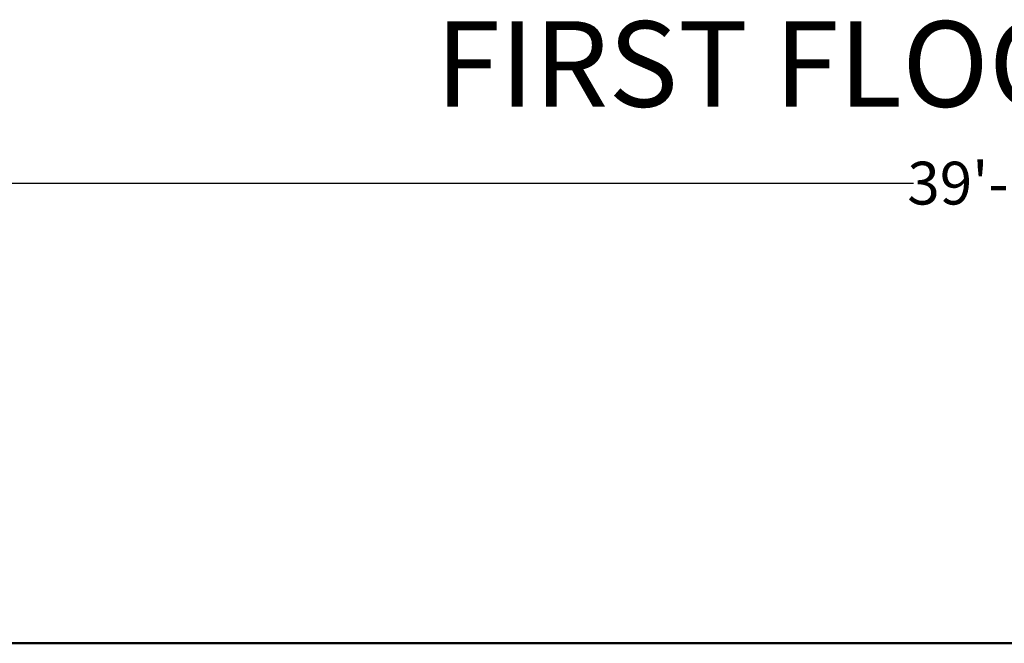
# Model space of a CAD drawing. Units: inches. Extents: x -173 to 545, y -746 to 104.
# Tile 30 of 32: x 125 to 263, y 17 to 104. Entities that reach past the tile are written whole.
import ezdxf

# ---------------------------------------------------------------- set-up
doc = ezdxf.new("R2010")
doc.units = ezdxf.units.IN
doc.header["$MEASUREMENT"] = 0
for name, color, linetype, lineweight in [('A-ANNO-DIMS', 2, 'Continuous', 18), ('A-ANNO-TEXT', 7, 'Continuous', 18), ('A-WALL', 7, 'Continuous', 50)]:
    doc.layers.add(name, color=color, linetype=linetype, lineweight=lineweight)
doc.styles.get("Standard").update_dxf_attribs({"font": 'arial.ttf'})
doc.dimstyles.get("Standard").update_dxf_attribs({"dimtxt": 0.18, "dimasz": 0.18, "dimexe": 0.18, "dimexo": 0.0625, "dimgap": 0.09, "dimtad": 0, "dimtih": 1, "dimtoh": 1, "dimdec": 0, "dimzin": 0, "dimdsep": 46, "dimlunit": 3, "dimtxsty": 'Standard', "dimcen": 0.09, "dimadec": 0, "dimazin": 0, "dimtfac": 1, "dimtdec": 0, "dimtofl": 0, "dimtmove": 0, "dimatfit": 3, "dimfxl": 1, "dimtolj": 1, "dimtzin": 0, "dimarcsym": 0})

# ---------------------------------------------------------------- blocks, each defined once
blk = doc.blocks.new('*D23')
at = {"layer": 'A-ANNO-DIMS', "color": 0, "lineweight": -2, "transparency": 16777216}
for p, q in [((24.3, 16.7), (24.3, 81.33)), ((24.48, 81.15), (250.33, 81.15)), ((501.62, 81.15), (275.78, 81.15)), ((501.8, 16.7), (501.8, 81.33))]:
    blk.add_line(p, q, dxfattribs=at)
at = {"layer": 'A-ANNO-DIMS', "color": 0, "transparency": 16777216}
for points in [[(24.48, 81.18), (24.48, 81.12), (24.3, 81.15)], [(501.62, 81.18), (501.62, 81.12), (501.8, 81.15)]]:
    blk.add_solid(points, dxfattribs=at)
at = {"layer": 'Defpoints', "color": 0, "transparency": 16777216}
for p in [(501.8, 81.15), (24.3, 16.64), (501.8, 16.64)]:
    blk.add_point(p, dxfattribs=at)
at = {"layer": 'A-ANNO-DIMS', "color": 0, "transparency": 16777216, "insert": (263.05, 81.15), "char_height": 6, "attachment_point": 5}
blk.add_mtext('\\A1;39\'-10"', dxfattribs=at)

msp = doc.modelspace()

# ---------------------------------------------------------------- linework, layer by layer
at = {"layer": 'A-WALL'}
msp.add_line((24.3, 16.64), (501.8, 16.64), dxfattribs=at)

# ---------------------------------------------------------------- texts
at = {"layer": 'A-ANNO-TEXT', "insert": (183.35, 103.85), "char_height": 12, "attachment_point": 1}
msp.add_mtext('FIRST FLOOR PLAN', dxfattribs=at)

# ---------------------------------------------------------------- dimensions: what is measured, and where the dimension line sits
at = {"layer": 'A-ANNO-DIMS'}
dim = msp.add_linear_dim(base=(501.80136521, 81.15311648), p1=(24.30136521, 16.63801408), p2=(501.80136521, 16.63801408), dimstyle='Standard', override={"dimtxt": 6, "dimclrd": 0, "dimclre": 0, "dimclrt": 0}, dxfattribs=at)
dim.commit()
dim.dimension.update_dxf_attribs({"geometry": '*D23', "text_midpoint": (263.05136521, 81.15311648)})

doc.saveas('drawing.dxf')
